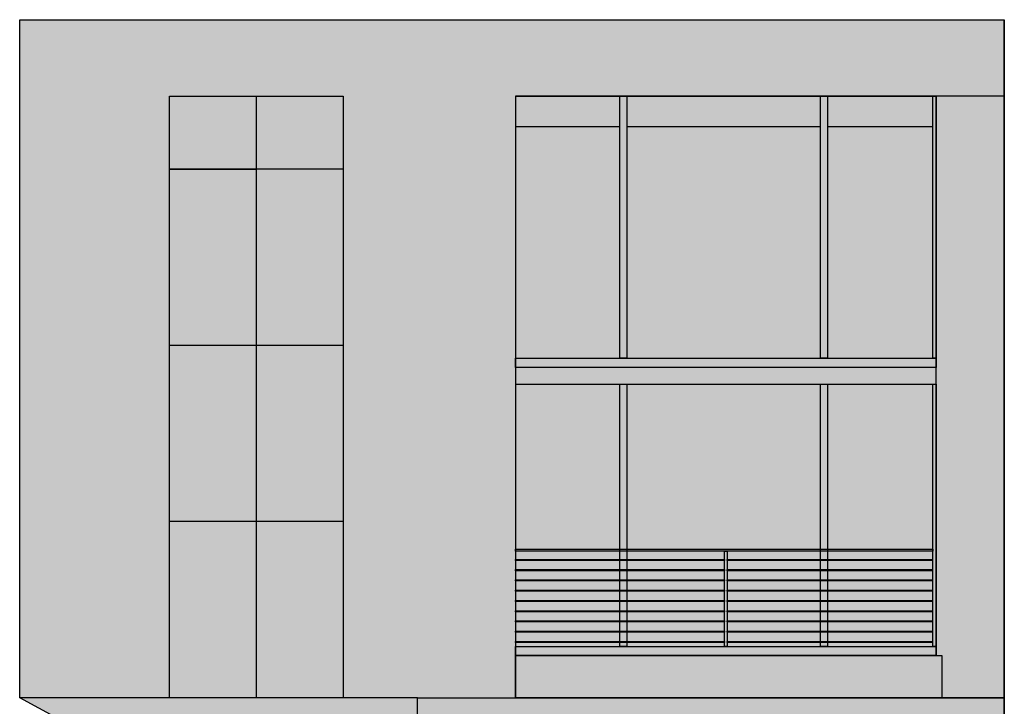
# Model space of a CAD drawing. Units: feet. Extents: x 2368 to 3224, y 836 to 1229.
# Tile 8 of 9: x 2368 to 2719, y 985 to 1229. Entities that reach past the tile are written whole.
import ezdxf

# ---------------------------------------------------------------- set-up
doc = ezdxf.new("R2010")
doc.units = ezdxf.units.FT
doc.layers.add('A-ELEV', color=7, linetype='Continuous', lineweight=25)
doc.layers.add('A-ELEV-PATT', color=8, linetype='Continuous', lineweight=13)

msp = doc.modelspace()

# ---------------------------------------------------------------- hatches: boundary and pattern name
at = {"layer": 'A-ELEV-PATT'}
h = msp.add_hatch(color=256, dxfattribs=at)
h.dxf.hatch_style = 1
h.paths.add_polyline_path([(2421.63, 1202.15), (2483.52, 1202.15), (2483.52, 987.86), (2510.02, 987.86), (2544.98, 987.86), (2544.98, 1002.87), (2544.98, 1006.11), (2544.98, 1202.15), (2719.16, 1202.15), (2719.16, 1229.35), (2368.3, 1229.35), (2368.3, 987.86), (2421.63, 987.86), (2421.63, 1050.6)])
h = msp.add_hatch(color=256, dxfattribs=at)
h.dxf.hatch_style = 1
h.paths.add_polyline_path([(2584.6, 1202.15), (2582.11, 1202.15), (2582.11, 1108.75), (2584.6, 1108.75)])
h.paths.add_polyline_path([(2656.21, 1202.15), (2653.72, 1202.15), (2653.72, 1108.75), (2656.21, 1108.75)])
h.paths.add_polyline_path([(2693.73, 1040.78), (2656.21, 1040.78), (2656.21, 1099.51), (2653.72, 1099.51), (2653.72, 1040.78), (2584.6, 1040.78), (2584.6, 1099.51), (2582.11, 1099.51), (2582.11, 1040.78), (2544.98, 1040.78), (2544.98, 1040.06), (2582.11, 1040.06), (2582.11, 1037.14), (2544.98, 1037.14), (2544.98, 1036.77), (2582.11, 1036.77), (2582.11, 1033.48), (2544.98, 1033.48), (2544.98, 1033.11), (2582.11, 1033.11), (2582.11, 1029.83), (2544.98, 1029.83), (2544.98, 1029.46), (2582.11, 1029.46), (2582.11, 1026.18), (2544.98, 1026.18), (2544.98, 1025.81), (2582.11, 1025.81), (2582.11, 1022.52), (2544.98, 1022.52), (2544.98, 1022.15), (2582.11, 1022.15), (2582.11, 1018.87), (2544.98, 1018.87), (2544.98, 1018.5), (2582.11, 1018.5), (2582.11, 1015.21), (2544.98, 1015.21), (2544.98, 1014.84), (2582.11, 1014.84), (2582.11, 1011.56), (2544.98, 1011.56), (2544.98, 1011.19), (2582.11, 1011.19), (2582.11, 1007.9), (2544.98, 1007.9), (2544.98, 1007.53), (2582.11, 1007.53), (2582.11, 1006.11), (2584.6, 1006.11), (2584.6, 1007.53), (2619.49, 1007.53), (2619.49, 1006.11), (2620.43, 1006.11), (2620.43, 1007.53), (2653.72, 1007.53), (2653.72, 1006.11), (2656.21, 1006.11), (2656.21, 1007.53), (2693.73, 1007.53), (2693.73, 1007.9), (2656.21, 1007.9), (2656.21, 1011.19), (2693.73, 1011.19), (2693.73, 1011.56), (2656.21, 1011.56), (2656.21, 1014.84), (2693.73, 1014.84), (2693.73, 1015.21), (2656.21, 1015.21), (2656.21, 1018.5), (2693.73, 1018.5), (2693.73, 1018.87), (2656.21, 1018.87), (2656.21, 1022.15), (2693.73, 1022.15), (2693.73, 1022.52), (2656.21, 1022.52), (2656.21, 1025.81), (2693.73, 1025.81), (2693.73, 1026.18), (2656.21, 1026.18), (2656.21, 1029.46), (2693.73, 1029.46), (2693.73, 1029.83), (2656.21, 1029.83), (2656.21, 1033.11), (2693.73, 1033.11), (2693.73, 1033.48), (2656.21, 1033.48), (2656.21, 1036.77), (2693.73, 1036.77), (2693.73, 1037.14), (2656.21, 1037.14), (2656.21, 1040.06), (2693.73, 1040.06)])
h.paths.add_polyline_path([(2584.6, 1040.06), (2619.49, 1040.06), (2619.49, 1037.14), (2584.6, 1037.14)], flags=16)
h.paths.add_polyline_path([(2584.6, 1036.77), (2619.49, 1036.77), (2619.49, 1033.48), (2584.6, 1033.48)], flags=16)
h.paths.add_polyline_path([(2584.6, 1033.11), (2619.49, 1033.11), (2619.49, 1029.83), (2584.6, 1029.83)], flags=16)
h.paths.add_polyline_path([(2584.6, 1029.46), (2619.49, 1029.46), (2619.49, 1026.18), (2584.6, 1026.18)], flags=16)
h.paths.add_polyline_path([(2584.6, 1025.81), (2619.49, 1025.81), (2619.49, 1022.52), (2584.6, 1022.52)], flags=16)
h.paths.add_polyline_path([(2584.6, 1022.15), (2619.49, 1022.15), (2619.49, 1018.87), (2584.6, 1018.87)], flags=16)
h.paths.add_polyline_path([(2584.6, 1018.5), (2619.49, 1018.5), (2619.49, 1015.21), (2584.6, 1015.21)], flags=16)
h.paths.add_polyline_path([(2584.6, 1014.84), (2619.49, 1014.84), (2619.49, 1011.56), (2584.6, 1011.56)], flags=16)
h.paths.add_polyline_path([(2584.6, 1011.19), (2619.49, 1011.19), (2619.49, 1007.9), (2584.6, 1007.9)], flags=16)
h.paths.add_polyline_path([(2620.43, 1040.06), (2653.72, 1040.06), (2653.72, 1037.14), (2620.43, 1037.14)], flags=16)
h.paths.add_polyline_path([(2620.43, 1036.77), (2653.72, 1036.77), (2653.72, 1033.48), (2620.43, 1033.48)], flags=16)
h.paths.add_polyline_path([(2620.43, 1033.11), (2653.72, 1033.11), (2653.72, 1029.83), (2620.43, 1029.83)], flags=16)
h.paths.add_polyline_path([(2620.43, 1029.46), (2653.72, 1029.46), (2653.72, 1026.18), (2620.43, 1026.18)], flags=16)
h.paths.add_polyline_path([(2620.43, 1025.81), (2653.72, 1025.81), (2653.72, 1022.52), (2620.43, 1022.52)], flags=16)
h.paths.add_polyline_path([(2620.43, 1022.15), (2653.72, 1022.15), (2653.72, 1018.87), (2620.43, 1018.87)], flags=16)
h.paths.add_polyline_path([(2620.43, 1018.5), (2653.72, 1018.5), (2653.72, 1015.21), (2620.43, 1015.21)], flags=16)
h.paths.add_polyline_path([(2620.43, 1014.84), (2653.72, 1014.84), (2653.72, 1011.56), (2620.43, 1011.56)], flags=16)
h.paths.add_polyline_path([(2620.43, 1011.19), (2653.72, 1011.19), (2653.72, 1007.9), (2620.43, 1007.9)], flags=16)
h.paths.add_polyline_path([(2536.7, 926.19), (2529.87, 926.19), (2529.87, 904.71), (2536.7, 904.71)])
h.paths.add_polyline_path([(2422.21, 920.11), (2416.4, 920.11), (2416.4, 905.78), (2422.21, 905.78)])
h = msp.add_hatch(color=256, dxfattribs=at)
h.dxf.hatch_style = 1
h.paths.add_polyline_path([(2452.58, 1176.09), (2421.63, 1176.09), (2421.63, 1113.35), (2452.58, 1113.35)])
h.paths.add_polyline_path([(2483.52, 1113.35), (2452.58, 1113.35), (2452.58, 1050.6), (2483.52, 1050.6)])
h.paths.add_polyline_path([(2452.58, 1050.6), (2421.63, 1050.6), (2421.63, 987.86), (2452.58, 987.86)])
h.paths.add_polyline_path([(2536.7, 926.19), (2536.7, 904.71), (2529.87, 904.71), (2529.87, 926.19)], flags=16)
h.paths.add_polyline_path([(2719.16, 1202.15), (2694.93, 1202.15), (2694.93, 1108.75), (2694.93, 1002.87), (2696.85, 1002.87), (2696.85, 987.86), (2719.16, 987.86)])
h = msp.add_hatch(color=256, dxfattribs=at)
h.dxf.hatch_style = 1
h.paths.add_polyline_path([(2452.58, 1202.15), (2421.63, 1202.15), (2421.63, 1176.09), (2452.58, 1176.09)])
h.paths.add_polyline_path([(2483.52, 1202.15), (2452.58, 1202.15), (2452.58, 1176.09), (2483.52, 1176.09)])
h.paths.add_polyline_path([(2483.52, 1176.09), (2452.58, 1176.09), (2452.58, 1113.35), (2483.52, 1113.35)])
h.paths.add_polyline_path([(2483.52, 1050.6), (2452.58, 1050.6), (2452.58, 987.86), (2483.52, 987.86)])
h.paths.add_polyline_path([(2452.58, 1113.35), (2421.63, 1113.35), (2421.63, 1050.6), (2452.58, 1050.6)])
h.paths.add_polyline_path([(2693.73, 1202.15), (2656.21, 1202.15), (2656.21, 1191.22), (2693.73, 1191.22)])
h.paths.add_polyline_path([(2653.72, 1202.15), (2584.6, 1202.15), (2584.6, 1191.22), (2653.72, 1191.22)])
h.paths.add_polyline_path([(2582.11, 1202.15), (2544.98, 1202.15), (2544.98, 1191.22), (2582.11, 1191.22)])
h = msp.add_hatch(dxfattribs=at)
h.set_pattern_fill('AR-PARQ1', color=256, scale=0.01)
h.paths.add_polyline_path([(2483.52, 1176.09), (2452.58, 1176.09), (2452.58, 1113.35), (2483.52, 1113.35)])
h.paths.add_polyline_path([(2452.58, 1202.15), (2421.63, 1202.15), (2421.63, 1176.09), (2452.58, 1176.09)])
h.paths.add_polyline_path([(2483.52, 1202.15), (2452.58, 1202.15), (2452.58, 1176.09), (2483.52, 1176.09)])
h.paths.add_polyline_path([(2452.58, 1113.35), (2421.63, 1113.35), (2421.63, 1050.6), (2452.58, 1050.6)])
h.paths.add_polyline_path([(2483.52, 1050.6), (2452.58, 1050.6), (2452.58, 987.86), (2458.33, 987.86), (2483.52, 987.86)])
h.paths.add_polyline_path([(2582.11, 1202.15), (2544.98, 1202.15), (2544.98, 1191.22), (2582.11, 1191.22)])
h.paths.add_polyline_path([(2653.72, 1202.15), (2584.6, 1202.15), (2584.6, 1191.22), (2653.72, 1191.22)])
h.paths.add_polyline_path([(2693.73, 1202.15), (2656.21, 1202.15), (2656.21, 1191.22), (2693.73, 1191.22)])
h = msp.add_hatch(color=256, dxfattribs=at)
h.dxf.hatch_style = 1
h.paths.add_polyline_path([(2694.93, 1105.51), (2544.98, 1105.51), (2544.98, 1099.51), (2694.93, 1099.51)])
h.paths.add_polyline_path([(2694.93, 1108.75), (2693.73, 1108.75), (2544.98, 1108.75), (2544.98, 1105.51), (2694.93, 1105.51)])
h.paths.add_polyline_path([(2694.93, 1202.15), (2693.73, 1202.15), (2693.73, 1108.75), (2694.93, 1108.75)])
h.paths.add_polyline_path([(2694.93, 1099.51), (2693.73, 1099.51), (2693.73, 1006.11), (2694.93, 1006.11)])
h.paths.add_polyline_path([(2696.85, 1002.87), (2544.98, 1002.87), (2544.98, 987.86), (2696.85, 987.86)])
h.paths.add_polyline_path([(2694.93, 1006.11), (2693.73, 1006.11), (2544.98, 1006.11), (2544.98, 1002.87), (2694.93, 1002.87)])
h = msp.add_hatch(color=256, dxfattribs=at)
h.dxf.hatch_style = 1
h.paths.add_polyline_path([(2582.11, 1191.22), (2544.98, 1191.22), (2544.98, 1108.75), (2582.11, 1108.75)])
h.paths.add_polyline_path([(2653.72, 1191.22), (2584.6, 1191.22), (2584.6, 1108.75), (2653.72, 1108.75)])
h.paths.add_polyline_path([(2693.73, 1191.22), (2656.21, 1191.22), (2656.21, 1108.75), (2693.73, 1108.75)])
h.paths.add_polyline_path([(2653.72, 1099.51), (2584.6, 1099.51), (2584.6, 1040.78), (2653.72, 1040.78)])
h.paths.add_polyline_path([(2693.73, 1099.51), (2656.21, 1099.51), (2656.21, 1040.78), (2693.73, 1040.78)])
h.paths.add_polyline_path([(2582.11, 1099.51), (2544.98, 1099.51), (2544.98, 1040.78), (2582.11, 1040.78)])
h.paths.add_polyline_path([(2582.11, 1036.77), (2544.98, 1036.77), (2544.98, 1033.48), (2582.11, 1033.48)])
h.paths.add_polyline_path([(2582.11, 1033.11), (2544.98, 1033.11), (2544.98, 1029.83), (2582.11, 1029.83)])
h.paths.add_polyline_path([(2582.11, 1029.46), (2544.98, 1029.46), (2544.98, 1026.18), (2582.11, 1026.18)])
h.paths.add_polyline_path([(2582.11, 1025.81), (2544.98, 1025.81), (2544.98, 1022.52), (2582.11, 1022.52)])
h.paths.add_polyline_path([(2582.11, 1022.15), (2544.98, 1022.15), (2544.98, 1018.87), (2582.11, 1018.87)])
h.paths.add_polyline_path([(2582.11, 1018.5), (2544.98, 1018.5), (2544.98, 1015.21), (2582.11, 1015.21)])
h.paths.add_polyline_path([(2582.11, 1007.53), (2544.98, 1007.53), (2544.98, 1006.11), (2582.11, 1006.11)])
h.paths.add_polyline_path([(2582.11, 1011.19), (2544.98, 1011.19), (2544.98, 1007.9), (2582.11, 1007.9)])
h.paths.add_polyline_path([(2582.11, 1014.84), (2544.98, 1014.84), (2544.98, 1011.56), (2582.11, 1011.56)])
h.paths.add_polyline_path([(2619.49, 1007.53), (2584.6, 1007.53), (2584.6, 1006.11), (2619.49, 1006.11)])
h.paths.add_polyline_path([(2619.49, 1011.19), (2584.6, 1011.19), (2584.6, 1007.9), (2619.49, 1007.9)])
h.paths.add_polyline_path([(2619.49, 1014.84), (2584.6, 1014.84), (2584.6, 1011.56), (2619.49, 1011.56)])
h.paths.add_polyline_path([(2619.49, 1018.5), (2584.6, 1018.5), (2584.6, 1015.21), (2619.49, 1015.21)])
h.paths.add_polyline_path([(2619.49, 1022.15), (2584.6, 1022.15), (2584.6, 1018.87), (2619.49, 1018.87)])
h.paths.add_polyline_path([(2619.49, 1025.81), (2584.6, 1025.81), (2584.6, 1022.52), (2619.49, 1022.52)])
h.paths.add_polyline_path([(2619.49, 1029.46), (2584.6, 1029.46), (2584.6, 1026.18), (2619.49, 1026.18)])
h.paths.add_polyline_path([(2619.49, 1033.11), (2584.6, 1033.11), (2584.6, 1029.83), (2619.49, 1029.83)])
h.paths.add_polyline_path([(2619.49, 1036.77), (2584.6, 1036.77), (2584.6, 1033.48), (2619.49, 1033.48)])
h.paths.add_polyline_path([(2582.11, 1040.06), (2544.98, 1040.06), (2544.98, 1037.14), (2582.11, 1037.14)])
h.paths.add_polyline_path([(2619.49, 1040.06), (2584.6, 1040.06), (2584.6, 1037.14), (2619.49, 1037.14)])
h.paths.add_polyline_path([(2653.72, 1040.06), (2620.43, 1040.06), (2620.43, 1037.14), (2653.72, 1037.14)])
h.paths.add_polyline_path([(2653.72, 1036.77), (2620.43, 1036.77), (2620.43, 1033.48), (2653.72, 1033.48)])
h.paths.add_polyline_path([(2653.72, 1033.11), (2620.43, 1033.11), (2620.43, 1029.83), (2653.72, 1029.83)])
h.paths.add_polyline_path([(2653.72, 1029.46), (2620.43, 1029.46), (2620.43, 1026.18), (2653.72, 1026.18)])
h.paths.add_polyline_path([(2653.72, 1025.81), (2620.43, 1025.81), (2620.43, 1022.52), (2653.72, 1022.52)])
h.paths.add_polyline_path([(2653.72, 1022.15), (2620.43, 1022.15), (2620.43, 1018.87), (2653.72, 1018.87)])
h.paths.add_polyline_path([(2653.72, 1018.5), (2620.43, 1018.5), (2620.43, 1015.21), (2653.72, 1015.21)])
h.paths.add_polyline_path([(2653.72, 1011.19), (2620.43, 1011.19), (2620.43, 1007.9), (2653.72, 1007.9)])
h.paths.add_polyline_path([(2653.72, 1014.84), (2620.43, 1014.84), (2620.43, 1011.56), (2653.72, 1011.56)])
h.paths.add_polyline_path([(2653.72, 1007.53), (2620.43, 1007.53), (2620.43, 1006.11), (2653.72, 1006.11)])
h.paths.add_polyline_path([(2693.73, 1007.53), (2656.21, 1007.53), (2656.21, 1006.11), (2693.73, 1006.11)])
h.paths.add_polyline_path([(2693.73, 1011.19), (2656.21, 1011.19), (2656.21, 1007.9), (2693.73, 1007.9)])
h.paths.add_polyline_path([(2693.73, 1014.84), (2656.21, 1014.84), (2656.21, 1011.56), (2693.73, 1011.56)])
h.paths.add_polyline_path([(2693.73, 1018.5), (2656.21, 1018.5), (2656.21, 1015.21), (2693.73, 1015.21)])
h.paths.add_polyline_path([(2693.73, 1022.15), (2656.21, 1022.15), (2656.21, 1018.87), (2693.73, 1018.87)])
h.paths.add_polyline_path([(2693.73, 1025.81), (2656.21, 1025.81), (2656.21, 1022.52), (2693.73, 1022.52)])
h.paths.add_polyline_path([(2693.73, 1029.46), (2656.21, 1029.46), (2656.21, 1026.18), (2693.73, 1026.18)])
h.paths.add_polyline_path([(2693.73, 1033.11), (2656.21, 1033.11), (2656.21, 1029.83), (2693.73, 1029.83)])
h.paths.add_polyline_path([(2693.73, 1040.06), (2656.21, 1040.06), (2656.21, 1037.14), (2693.73, 1037.14)])
h.paths.add_polyline_path([(2693.73, 1036.77), (2656.21, 1036.77), (2656.21, 1033.48), (2693.73, 1033.48)])
h.paths.add_polyline_path([(2510.02, 968.65), (2451.35, 968.65), (2451.35, 916.99), (2510.02, 916.99)])
h.paths.add_polyline_path([(2510.02, 916.99), (2470.8, 916.99), (2470.8, 861.76), (2510.02, 861.76)])
h.paths.add_polyline_path([(2650.82, 971.36, 0.250141), (2603.19, 971.36), (2603.19, 926.73), (2650.82, 926.73)])
h.paths.add_polyline_path([(2651.5, 971), (2651.5, 926.73), (2677.6, 926.73, 0.272847)])
h.paths.add_polyline_path([(2677.6, 926.06), (2651.5, 926.06), (2651.5, 854.24), (2677.6, 854.24)])
h.paths.add_polyline_path([(2650.82, 926.06), (2603.19, 926.06), (2603.19, 854.24), (2650.82, 854.24)])
h.paths.add_polyline_path([(2602.51, 971, 0.272847), (2576.42, 926.73), (2602.51, 926.73)])
h.paths.add_polyline_path([(2602.51, 926.06), (2576.42, 926.06), (2576.42, 854.24), (2602.51, 854.24)])
h = msp.add_hatch(color=256, dxfattribs=at)
h.dxf.hatch_style = 1
h.paths.add_polyline_path([(2443.04, 973.51), (2394.91, 973.51), (2394.91, 853.51), (2443.04, 853.51)])
h.paths.add_polyline_path([(2422.21, 920.11), (2422.21, 905.78), (2416.4, 905.78), (2416.4, 920.11)], flags=16)
h.paths.add_polyline_path([(2449.3, 970.69), (2443.04, 973.51), (2443.04, 853.51), (2449.3, 853.51)])
h.paths.add_polyline_path([(2510.02, 987.86), (2368.3, 987.86), (2394.91, 973.51), (2443.04, 973.51), (2510.02, 973.51)])
h.paths.add_polyline_path([(2510.02, 973.51), (2443.04, 973.51), (2449.3, 970.69), (2510.02, 970.69)])
h = msp.add_hatch(color=256, dxfattribs=at)
h.dxf.hatch_style = 1
h.paths.add_polyline_path([(2624.92, 981.22), (2624.92, 981.73, -0.018787), (2629.09, 981.73), (2629.09, 981.22, -0.403049), (2681.53, 926.73), (2681.53, 853.51), (2701.14, 853.51), (2719.16, 853.51), (2719.16, 987.86), (2694.93, 987.86), (2544.98, 987.86), (2510.02, 987.86), (2510.02, 853.51), (2520.58, 853.51), (2520.05, 853.96), (2521, 855.17), (2521.51, 855.27), (2521.73, 855.83), (2522.31, 855.46), (2523.63, 855.92), (2523.84, 857.04), (2523.12, 857.51), (2521.95, 857.23), (2522.6, 858.63), (2522.68, 858.26), (2523.55, 858.73), (2524.28, 859.19), (2524.94, 859.29), (2525.23, 860.22), (2524.5, 860.32), (2525.17, 860.97), (2525.74, 860.88), (2525.67, 861.62), (2525.16, 861.72), (2525.3, 862.09), (2525.67, 862.19), (2526.32, 861.72), (2526.98, 862.19), (2526.47, 863.03), (2526.98, 863.31), (2526.98, 863.59), (2528.51, 865.09), (2528.51, 865.74), (2528.95, 866.58), (2529.53, 866.48), (2530.04, 866.95), (2530.41, 866.77), (2530.48, 866.3), (2530.77, 866.11), (2531.28, 866.67), (2531.86, 866.03), (2532.01, 864.99), (2533.1, 863.68), (2532.52, 863.68), (2532.3, 862.65), (2532.67, 861.9), (2533.18, 861.9), (2533.61, 862), (2534.34, 860.41), (2534.71, 860.41), (2535.29, 858.63), (2534.63, 857.61), (2536.09, 857.14), (2537.26, 855.92), (2536.52, 854.02), (2536.97, 853.96), (2537.09, 853.51), (2572.48, 853.51), (2572.48, 926.73, -0.403049)])
h.paths.add_polyline_path([(2536.7, 926.19), (2536.7, 904.71), (2529.87, 904.71), (2529.87, 926.19)], flags=16)

# ---------------------------------------------------------------- linework, layer by layer
at = {"layer": 'A-ELEV'}
for p, q in [((2368.3, 987.86), (2368.3, 1229.35)), ((2368.3, 987.86), (2368.3, 1229.35)), ((2719.16, 853.51), (2719.16, 1229.35)), ((2719.16, 853.51), (2719.16, 1229.35)), ((2452.58, 1202.15), (2452.58, 987.86)), ((2452.58, 1202.15), (2452.58, 987.86)), ((2544.98, 1202.15), (2694.93, 1202.15)), ((2544.98, 1202.15), (2694.93, 1202.15)), ((2582.11, 1191.22), (2544.98, 1191.22)), ((2582.11, 1191.22), (2544.98, 1191.22)), ((2653.72, 1191.22), (2584.6, 1191.22)), ((2653.72, 1191.22), (2584.6, 1191.22)), ((2693.73, 1191.22), (2656.21, 1191.22)), ((2693.73, 1191.22), (2656.21, 1191.22)), ((2483.52, 1176.09), (2421.63, 1176.09)), ((2483.52, 1176.09), (2421.63, 1176.09)), ((2694.93, 1105.51), (2544.98, 1105.51)), ((2694.93, 1105.51), (2544.98, 1105.51)), ((2544.98, 1099.51), (2694.93, 1099.51)), ((2544.98, 1099.51), (2694.93, 1099.51)), ((2510.02, 987.86), (2368.3, 987.86)), ((2394.91, 973.51), (2368.3, 987.86)), ((2510.02, 987.86), (2368.3, 987.86)), ((2394.91, 973.51), (2368.3, 987.86))]:
    msp.add_line(p, q, dxfattribs=at)
for points in [[(2368.3, 1229.35), (2719.16, 1229.35), (2719.16, 1202.15), (2544.98, 1202.15)], [(2368.3, 1229.35), (2719.16, 1229.35), (2719.16, 1202.15), (2544.98, 1202.15)], [(2719.16, 1229.35), (2719.16, 987.86), (2694.93, 987.86)], [(2719.16, 1229.35), (2719.16, 987.86), (2694.93, 987.86)], [(2544.98, 1202.15), (2544.98, 987.86)], [(2544.98, 1202.15), (2544.98, 987.86)], [(2694.93, 1002.87), (2694.93, 1202.15)], [(2694.93, 1002.87), (2694.93, 1202.15)], [(2483.52, 1113.35), (2421.63, 1113.35), (2421.63, 1176.09), (2452.58, 1176.09)], [(2483.52, 1113.35), (2421.63, 1113.35), (2421.63, 1176.09), (2452.58, 1176.09)], [(2483.52, 1113.35), (2483.52, 1050.6), (2421.63, 1050.6)], [(2483.52, 1113.35), (2483.52, 1050.6), (2421.63, 1050.6)], [(2458.33, 987.86), (2421.63, 987.86), (2421.63, 1050.6)], [(2458.33, 987.86), (2421.63, 987.86), (2421.63, 1050.6)], [(2693.73, 1036.77), (2620.43, 1036.77), (2620.43, 1037.14), (2693.73, 1037.14)], [(2693.73, 1036.77), (2620.43, 1036.77), (2620.43, 1037.14), (2693.73, 1037.14)], [(2694.93, 1037.14), (2694.93, 1036.77)], [(2694.93, 1037.14), (2694.93, 1036.77)], [(2693.73, 1033.11), (2620.43, 1033.11), (2620.43, 1033.48), (2693.73, 1033.48)], [(2693.73, 1033.11), (2620.43, 1033.11), (2620.43, 1033.48), (2693.73, 1033.48)], [(2694.93, 1033.48), (2694.93, 1033.11)], [(2694.93, 1033.48), (2694.93, 1033.11)], [(2693.73, 1029.46), (2620.43, 1029.46), (2620.43, 1029.83), (2693.73, 1029.83)], [(2693.73, 1029.46), (2620.43, 1029.46), (2620.43, 1029.83), (2693.73, 1029.83)], [(2694.93, 1029.83), (2694.93, 1029.46)], [(2694.93, 1029.83), (2694.93, 1029.46)], [(2693.73, 1025.81), (2620.43, 1025.81), (2620.43, 1026.18), (2693.73, 1026.18)], [(2693.73, 1025.81), (2620.43, 1025.81), (2620.43, 1026.18), (2693.73, 1026.18)], [(2694.93, 1026.18), (2694.93, 1025.81)], [(2694.93, 1026.18), (2694.93, 1025.81)], [(2693.73, 1022.15), (2620.43, 1022.15), (2620.43, 1022.52), (2693.73, 1022.52)], [(2693.73, 1022.15), (2620.43, 1022.15), (2620.43, 1022.52), (2693.73, 1022.52)], [(2694.93, 1022.52), (2694.93, 1022.15)], [(2694.93, 1022.52), (2694.93, 1022.15)], [(2693.73, 1018.5), (2620.43, 1018.5), (2620.43, 1018.87), (2693.73, 1018.87)], [(2693.73, 1018.5), (2620.43, 1018.5), (2620.43, 1018.87), (2693.73, 1018.87)], [(2694.93, 1018.87), (2694.93, 1018.5)], [(2694.93, 1018.87), (2694.93, 1018.5)], [(2693.73, 1014.84), (2620.43, 1014.84), (2620.43, 1015.21), (2693.73, 1015.21)], [(2693.73, 1014.84), (2620.43, 1014.84), (2620.43, 1015.21), (2693.73, 1015.21)], [(2694.93, 1015.21), (2694.93, 1014.84)], [(2694.93, 1015.21), (2694.93, 1014.84)], [(2693.73, 1011.19), (2620.43, 1011.19), (2620.43, 1011.56), (2693.73, 1011.56)], [(2693.73, 1011.19), (2620.43, 1011.19), (2620.43, 1011.56), (2693.73, 1011.56)], [(2694.93, 1011.56), (2694.93, 1011.19)], [(2694.93, 1011.56), (2694.93, 1011.19)], [(2693.73, 1007.53), (2620.43, 1007.53), (2620.43, 1007.9), (2693.73, 1007.9)], [(2693.73, 1007.53), (2620.43, 1007.53), (2620.43, 1007.9), (2693.73, 1007.9)], [(2694.93, 1007.9), (2694.93, 1007.53)], [(2694.93, 1007.9), (2694.93, 1007.53)], [(2521.04, 853.51), (2510.02, 853.51), (2510.02, 987.86), (2719.16, 987.86), (2719.16, 853.51), (2537.09, 853.51)], [(2521.04, 853.51), (2510.02, 853.51), (2510.02, 987.86), (2719.16, 987.86), (2719.16, 853.51), (2537.09, 853.51)]]:
    msp.add_lwpolyline(points, dxfattribs=at)
for points in [[(2368.3, 1202.15), (2368.3, 1202.15)], [(2483.52, 987.86), (2421.63, 987.86), (2421.63, 1202.15), (2483.52, 1202.15)], [(2483.52, 987.86), (2421.63, 987.86), (2421.63, 1202.15), (2483.52, 1202.15)], [(2582.11, 1202.15), (2584.6, 1202.15), (2584.6, 1108.75), (2582.11, 1108.75)], [(2582.11, 1202.15), (2584.6, 1202.15), (2584.6, 1108.75), (2582.11, 1108.75)], [(2653.72, 1202.15), (2656.21, 1202.15), (2656.21, 1108.75), (2653.72, 1108.75)], [(2653.72, 1202.15), (2656.21, 1202.15), (2656.21, 1108.75), (2653.72, 1108.75)], [(2694.93, 1108.75), (2693.73, 1108.75), (2693.73, 1202.15), (2694.93, 1202.15)], [(2694.93, 1108.75), (2693.73, 1108.75), (2693.73, 1202.15), (2694.93, 1202.15)], [(2694.93, 1105.51), (2544.98, 1105.51), (2544.98, 1108.75), (2694.93, 1108.75)], [(2694.93, 1105.51), (2544.98, 1105.51), (2544.98, 1108.75), (2694.93, 1108.75)], [(2582.11, 1099.51), (2584.6, 1099.51), (2584.6, 1006.11), (2582.11, 1006.11)], [(2582.11, 1099.51), (2584.6, 1099.51), (2584.6, 1006.11), (2582.11, 1006.11)], [(2653.72, 1099.51), (2656.21, 1099.51), (2656.21, 1006.11), (2653.72, 1006.11)], [(2653.72, 1099.51), (2656.21, 1099.51), (2656.21, 1006.11), (2653.72, 1006.11)], [(2694.93, 1006.11), (2693.73, 1006.11), (2693.73, 1099.51), (2694.93, 1099.51)], [(2694.93, 1006.11), (2693.73, 1006.11), (2693.73, 1099.51), (2694.93, 1099.51)], [(2693.73, 1040.06), (2544.98, 1040.06), (2544.98, 1040.78), (2693.73, 1040.78)], [(2693.73, 1040.06), (2544.98, 1040.06), (2544.98, 1040.78), (2693.73, 1040.78)], [(2619.49, 1040.06), (2620.43, 1040.06), (2620.43, 1006.11), (2619.49, 1006.11)], [(2619.49, 1040.06), (2620.43, 1040.06), (2620.43, 1006.11), (2619.49, 1006.11)], [(2544.98, 1037.14), (2619.49, 1037.14), (2619.49, 1036.77), (2544.98, 1036.77)], [(2544.98, 1037.14), (2619.49, 1037.14), (2619.49, 1036.77), (2544.98, 1036.77)], [(2544.98, 1033.48), (2619.49, 1033.48), (2619.49, 1033.11), (2544.98, 1033.11)], [(2544.98, 1033.48), (2619.49, 1033.48), (2619.49, 1033.11), (2544.98, 1033.11)], [(2544.98, 1029.83), (2619.49, 1029.83), (2619.49, 1029.46), (2544.98, 1029.46)], [(2544.98, 1029.83), (2619.49, 1029.83), (2619.49, 1029.46), (2544.98, 1029.46)], [(2544.98, 1026.18), (2619.49, 1026.18), (2619.49, 1025.81), (2544.98, 1025.81)], [(2544.98, 1026.18), (2619.49, 1026.18), (2619.49, 1025.81), (2544.98, 1025.81)], [(2544.98, 1022.52), (2619.49, 1022.52), (2619.49, 1022.15), (2544.98, 1022.15)], [(2544.98, 1022.52), (2619.49, 1022.52), (2619.49, 1022.15), (2544.98, 1022.15)], [(2544.98, 1018.87), (2619.49, 1018.87), (2619.49, 1018.5), (2544.98, 1018.5)], [(2544.98, 1018.87), (2619.49, 1018.87), (2619.49, 1018.5), (2544.98, 1018.5)], [(2544.98, 1015.21), (2619.49, 1015.21), (2619.49, 1014.84), (2544.98, 1014.84)], [(2544.98, 1015.21), (2619.49, 1015.21), (2619.49, 1014.84), (2544.98, 1014.84)], [(2544.98, 1011.56), (2619.49, 1011.56), (2619.49, 1011.19), (2544.98, 1011.19)], [(2544.98, 1011.56), (2619.49, 1011.56), (2619.49, 1011.19), (2544.98, 1011.19)], [(2544.98, 1007.9), (2619.49, 1007.9), (2619.49, 1007.53), (2544.98, 1007.53)], [(2544.98, 1007.9), (2619.49, 1007.9), (2619.49, 1007.53), (2544.98, 1007.53)], [(2694.93, 1002.87), (2544.98, 1002.87), (2544.98, 1006.11), (2694.93, 1006.11)], [(2694.93, 1002.87), (2544.98, 1002.87), (2544.98, 1006.11), (2694.93, 1006.11)], [(2544.98, 1002.87), (2696.85, 1002.87), (2696.85, 987.86), (2544.98, 987.86)], [(2544.98, 1002.87), (2696.85, 1002.87), (2696.85, 987.86), (2544.98, 987.86)]]:
    msp.add_lwpolyline(points, close=True, dxfattribs=at)

doc.saveas('drawing.dxf')
